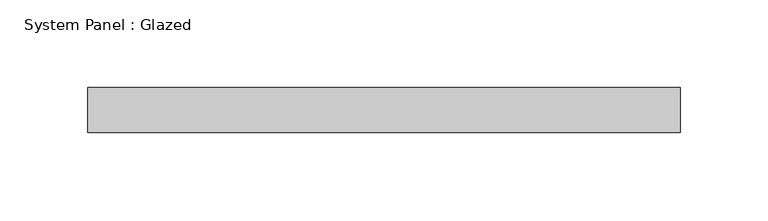
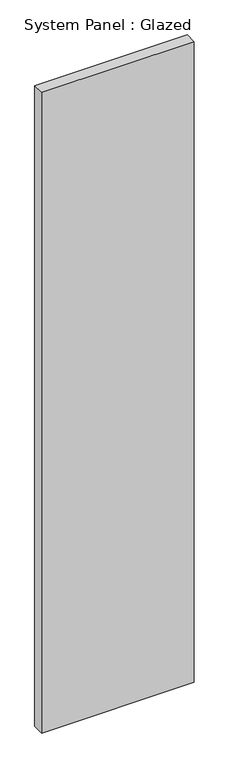
"""IFC4 building model written with IfcOpenShell, lengths in millimetres: plate geometry, System Panel : Glazed."""

from ifc_helpers import new_model, si_unit, origin, origin_with_axes, place, context, project, spatial, polyline, outline, extrude, source, transform, mapped, element, save


def system_panel_glazed_ed2eb233(model_context):
    return source(origin(), model_context, "Body", "SweptSolid", [
        extrude(outline(polyline([(168.275, 19.05), (-168.275, 19.05), (-168.275, 44.45), (168.275, 44.45), (168.275, 19.05)])), origin_with_axes(), (0.0, 0.0, 1.0), 1492.7840707),
    ])


if __name__ == "__main__":
    model = new_model("IFC4")
    model_context = context("Model", 3, world=origin())
    ifc_project = project(units=[si_unit("LENGTHUNIT", "METRE", prefix="MILLI")], contexts=[model_context])
    site = spatial("IfcSite", under=ifc_project)
    building = spatial("IfcBuilding", under=site)
    placement = place(None, origin())
    system_panel_glazed_shape = system_panel_glazed_ed2eb233(model_context)
    element("IfcPlate", 1, ObjectType="System Panel : Glazed", at=placement, inside=building, context=model_context, shape_type="MappedRepresentation", body=[
        mapped(system_panel_glazed_shape, transform((0.0, 0.0, 0.0), x_axis=(1.0, 0.0, 0.0), y_axis=(0.0, 1.0, 0.0), z_axis=(0.0, 0.0, 1.0))),
    ])
    save(model, "model.ifc")

# Revit data of these elements
# Type "System Panel : Glazed"
#   Construction Type Id = "GSP4R"
#   Analytic Construction = "1/8 in Pilkington single glazing"
#   Visual Light Transmittance = 0.9
#   Solar Heat Gain Coefficient = 0.86
#   Heat Transfer Coefficient (U) = 1.18115 BTU/(h·ft²·°F)
#   Define Thermal Properties by = 1
# Element 1 (IfcPlate, "System Panel : Glazed")
#   Materials on its faces: "Glass"
# Materials
#   "Glass": class "Glass", colour RGB 0 128 192, transparency 0.75, Description = "Soda Lime Glass", Cost = 0
